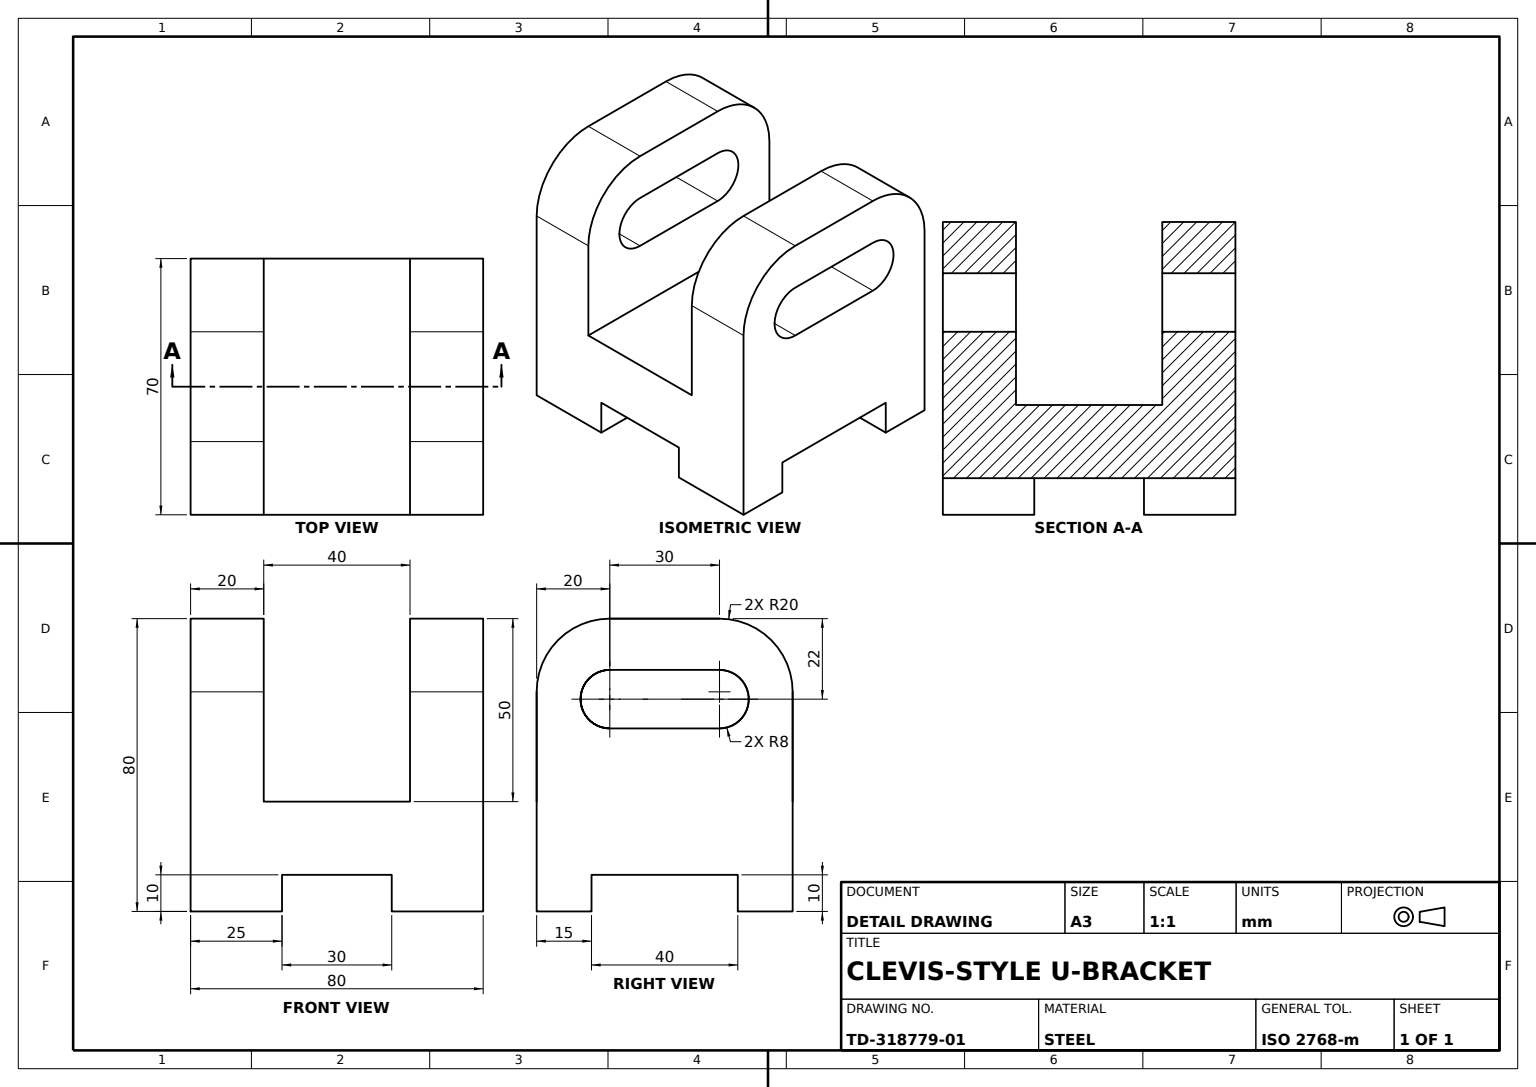
SolidWorks part; units mm, degrees
material "Plain Carbon Steel"
ref_plane "Front Plane" through (0, 0, 0) normal (0, 0, 1) x (1, 0, 0)
ref_plane "Top Plane" through (0, 0, 0) normal (0, 1, 0) x (1, 0, 0)
ref_plane "Right Plane" through (0, 0, 0) normal (1, 0, 0) x (0, 0, -1)
sketch "Base Block Profile 80x80" plane through (0, 0, 0) normal (1, 0, 0) x (0, 0, -1)
  line L1 (-40, 40) -> (40, 40)
  line L2 (-40, 40) -> (-40, -40)
  line L3 (-40, -40) -> (40, -40)
  line L4 (40, 40) -> (40, -40)
  line L5 (-40, 40) -> (40, -40) construction
  line L6 (-40, -40) -> (40, 40) construction
  point P0 (0, 0)
  dimension "D1" = 80
  dimension "D2" = 80
extrude "Base Block 80x80x70" add sketch "Base Block Profile 80x80" along normal mid plane 70
sketch "Notch Profile 20x20" plane through (35, 0, 0) normal (1, 0, 0) x (0, 0, -1)
  line L0 (40, 40) -> (-40, 40) construction
  line L1 (-20, 40) -> (20, 40)
  line L2 (-20, 40) -> (-20, -10)
  line L3 (-20, -10) -> (20, -10)
  line L4 (20, 40) -> (20, -10)
  line L5 (-40, 40) -> (-40, -40) construction
  line L6 (40, -40) -> (40, 40) construction
  dimension "D1" = 20
  dimension "D2" = 20
  dimension "D3" = 40
  dimension "D4" = 50
extrude "Notch Cut 20x20" cut sketch "Notch Profile 20x20" against normal through all both contours L2 L1 L4 L3
sketch "Notch Profile 25x25" plane through (35, 0, 0) normal (1, 0, 0) x (0, 0, -1)
  line L0 (-40, -40) -> (40, -40) construction
  line L1 (-15, -40) -> (15, -40)
  line L2 (-15, -40) -> (-15, -30)
  line L3 (-15, -30) -> (15, -30)
  line L4 (15, -40) -> (15, -30)
  line L5 (-40, 40) -> (-40, -40) construction
  line L6 (40, -40) -> (40, 40) construction
  dimension "D1" = 25
  dimension "D2" = 25
  dimension "D3" = 10
extrude "Notch Cut 25x25" cut sketch "Notch Profile 25x25" against normal through all both contours L2 L1 L4 L3
sketch "Pocket Profile 40x15" plane through (0, 0, 40) normal (0, 0, 1) x (1, 0, 0)
  line L0 (35, -40) -> (-35, -40) construction
  line L1 (-20, -40) -> (20, -40)
  line L2 (-20, -40) -> (-20, -30)
  line L3 (-20, -30) -> (20, -30)
  line L4 (20, -40) -> (20, -30)
  line L5 (-35, 40) -> (-35, -40) construction
  line L6 (35, 40) -> (35, -40) construction
  dimension "D1" = 40
  dimension "D2" = 15
  dimension "D3" = 15
  dimension "D4" = 10
extrude "Pocket Cut 40x15" cut sketch "Pocket Profile 40x15" against normal through all both
sketch "Upright Slot Profile" plane through (0, 0, 40) normal (0, 0, 1) x (1, 0, 0)
  line L0 (-49.5747, 18) -> (44.2704, 18) construction
  line L1 (35, 40) -> (-35, 40) construction
  line L2 (0, 0) -> (0, 49.7787) construction
  line L5 (-15, 18) -> (15, 18) construction
  line L6 (-15, 26) -> (15, 26)
  line L7 (-15, 10) -> (15, 10)
  arc A0 (-15, 26) -> (-15, 10) centre (-15, 18) ccw
  arc A1 (15, 10) -> (15, 26) centre (15, 18) ccw
  point P13 (0, 18)
  dimension "D4" = 8
  dimension "D5" = 18
  dimension "D1" = 22
  dimension "D2" = 15
  dimension "D3" = 30
extrude "Upright Slot Cut" cut sketch "Upright Slot Profile" against normal through all both
fillet "Upright Top Fillets R20" radius 20 4 edges at (-35, 40, 30) (-35, 40, -30) (35, 40, -30) (35, 40, 30)
